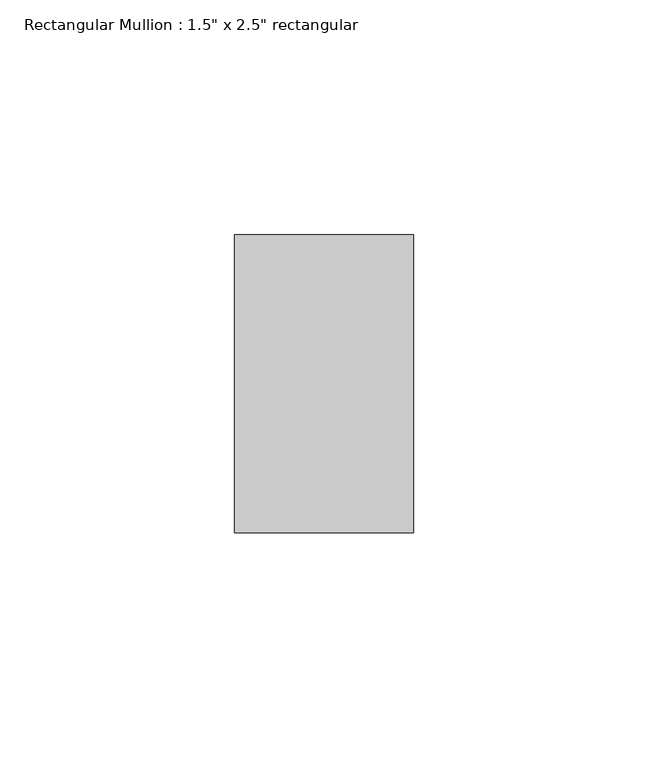
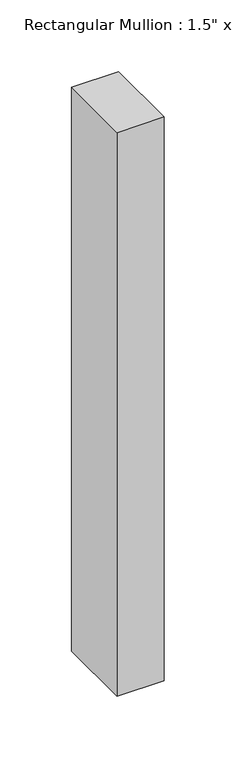
"""IFC4 building model written with IfcOpenShell, lengths in millimetres: member geometry."""

from ifc_helpers import new_model, si_unit, frame, origin, place, context, project, spatial, polyline, outline, extrude, source, transform, mapped, element, save


def member_ade56e03(model_context):
    return source(origin(), model_context, "Body", "SweptSolid", [
        extrude(outline(polyline([(0.0, 31.75), (0.0, -31.75), (-38.1, -31.75), (-38.1, 31.75), (0.0, 31.75)])), frame((0.0, 0.0, -480.1854569), z_axis=(0.0, 0.0, 1.0), x_axis=(1.0, 0.0, 0.0)), (0.0, 0.0, 1.0), 480.1854569),
    ])


if __name__ == "__main__":
    model = new_model("IFC4")
    model_context = context("Model", 3, world=origin())
    ifc_project = project(units=[si_unit("LENGTHUNIT", "METRE", prefix="MILLI")], contexts=[model_context])
    site = spatial("IfcSite", under=ifc_project)
    building = spatial("IfcBuilding", under=site)
    placement = place(None, origin())
    member_shape = member_ade56e03(model_context)
    element("IfcMember", 1, ObjectType="Rectangular Mullion : 1.5\" x 2.5\" rectangular", at=placement, inside=building, context=model_context, shape_type="MappedRepresentation", body=[
        mapped(member_shape, transform((0.0, 0.0, 0.0), x_axis=(1.0, 0.0, 0.0), y_axis=(0.0, 1.0, 0.0), z_axis=(0.0, 0.0, 1.0))),
    ])
    save(model, "model.ifc")

# Revit data of these elements
# Type "Rectangular Mullion : 1.5\" x 2.5\" rectangular"
#   built-in parameter 1007304 = 0.208333 (stored number, unit not read)
#   built-in parameter 1007301 = 0.0625 (stored number, unit not read)
#   built-in parameter 1007300 = 0.0625 (stored number, unit not read)
# Element 1 (IfcMember, "Rectangular Mullion : 1.5\" x 2.5\" rectangular")
#   Materials on its faces: "Leather - Black"
# Materials
#   "Leather - Black": class "Generic", colour RGB 40 40 40, transparency 0, Cost = 0
